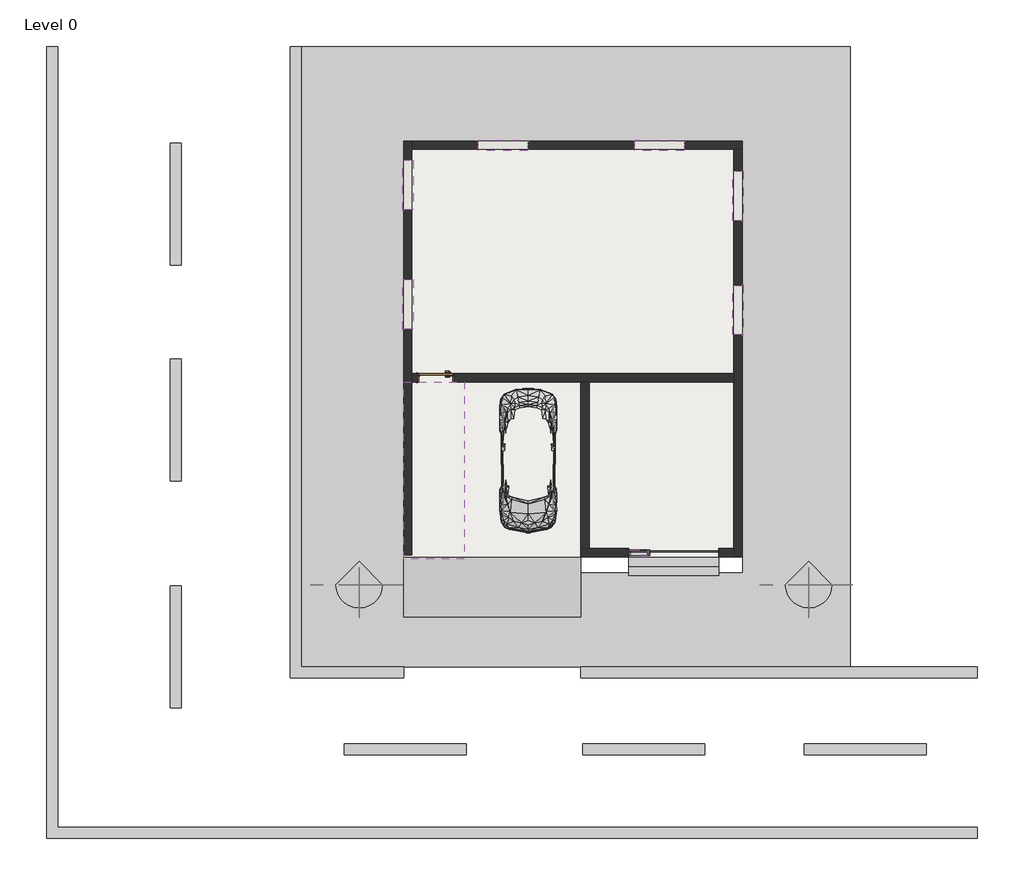
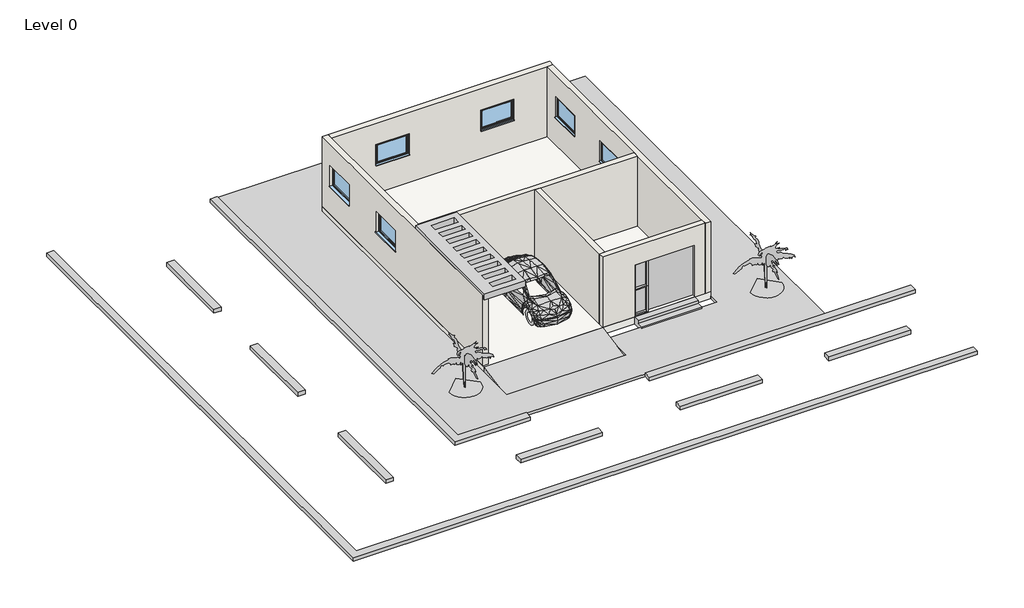
# One storey: 7 members, 6 walls, 6 windows, 4 proxies, 3 plates, 2 geographic elements, 1 door, 1 slab.
"""IFC4 building model written with IfcOpenShell, lengths in millimetres."""

from ifc_helpers import new_model, si_unit, frame, origin, origin_with_axes, place, context, project, spatial, polyline, outline, extrude, faceted_brep, transform, mapped, element, save
from components import generic_models_1_generic_models_1_b1455ff5, generic_models_4_generic_models_4_16c068d2, generic_models_5_generic_models_5_f3326099, rpc_beetle_rpc_beetle_31f8b51e, doors_intsgl_1010x2110mm_2294229c, rpc_tree_tropical_australian_tree_furn_6_77f1a640, rectangular_mullion_50x150mm_bddf6eb5, rectangular_mullion_50x150mm_e26dd5f5, rectangular_mullion_50x150mm_60451361, system_panel_glazed_79c163db, system_panel_glazed_e26c2a08, windows_sgl_plain_1360x910mm_0a0c3bd6

model = new_model("IFC4")

# Units and contexts
model_context = context("Model", 3, world=origin())
ifc_project = project(units=[si_unit("LENGTHUNIT", "METRE", prefix="MILLI")], contexts=[model_context])

# Site, building, storey
site = spatial("IfcSite", under=ifc_project)
building = spatial("IfcBuilding", under=site)
storey = spatial("IfcBuildingStorey", under=building, Name="Level 0", Elevation=0.0)

# Proxies
placement = place(None, origin())
generic_models_1_generic_models_1_shape = generic_models_1_generic_models_1_b1455ff5(model_context)
element("IfcBuildingElementProxy", 1, Name="Generic Models 1 : Generic Models 1", ObjectType="Generic Models 1 : Generic Models 1", at=placement, inside=storey, context=model_context, shape_type="MappedRepresentation", body=[
    mapped(generic_models_1_generic_models_1_shape, transform((0.0, 0.0, 0.0), x_axis=(1.0, 0.0, 0.0), y_axis=(0.0, 1.0, 0.0), z_axis=(0.0, 0.0, 1.0))),
])
generic_models_4_generic_models_4_shape = generic_models_4_generic_models_4_16c068d2(model_context)
element("IfcBuildingElementProxy", 2, Name="Generic Models 4 : Generic Models 4", ObjectType="Generic Models 4 : Generic Models 4", at=placement, inside=storey, context=model_context, shape_type="MappedRepresentation", body=[
    mapped(generic_models_4_generic_models_4_shape, transform((0.0, 0.0, 0.0), x_axis=(1.0, 0.0, 0.0), y_axis=(0.0, 1.0, 0.0), z_axis=(0.0, 0.0, 1.0))),
])
generic_models_5_generic_models_5_shape = generic_models_5_generic_models_5_f3326099(model_context)
element("IfcBuildingElementProxy", 3, Name="Generic Models 5 : Generic Models 5", ObjectType="Generic Models 5 : Generic Models 5", at=placement, inside=storey, context=model_context, shape_type="MappedRepresentation", body=[
    mapped(generic_models_5_generic_models_5_shape, transform((0.0, 0.0, 0.0), x_axis=(1.0, 0.0, 0.0), y_axis=(0.0, 1.0, 0.0), z_axis=(0.0, 0.0, 1.0))),
])
rpc_beetle_rpc_beetle_shape = rpc_beetle_rpc_beetle_31f8b51e(model_context)
element("IfcBuildingElementProxy", 4, Name="RPC Beetle : RPC Beetle", ObjectType="RPC Beetle : RPC Beetle", at=placement, inside=storey, context=model_context, shape_type="MappedRepresentation", body=[
    mapped(rpc_beetle_rpc_beetle_shape, transform((-6051.9025595, 647.0632107, 0.0), x_axis=(-1.0, 0.0, 0.0), y_axis=(0.0, -1.0, 0.0), z_axis=(0.0, 0.0, 1.0))),
])

# Door
doors_intsgl_1010x2110mm_shape = doors_intsgl_1010x2110mm_2294229c(model_context)
element("IfcDoor", 5, ObjectType="Doors_IntSgl : 1010x2110mm", at=placement, inside=storey, context=model_context, shape_type="MappedRepresentation", body=[
    mapped(doors_intsgl_1010x2110mm_shape, transform((-8594.9025595, 1694.8132107, 0.0), x_axis=(-1.0, 0.0, 0.0), y_axis=(0.0, -1.0, 0.0), z_axis=(0.0, 0.0, 1.0))),
])

# Geographic elements
rpc_tree_tropical_australian_tree_furn_6_shape = rpc_tree_tropical_australian_tree_furn_6_77f1a640(model_context)
element("IfcGeographicElement", 6, ObjectType="RPC Tree - Tropical : Australian Tree Furn - 6'", at=placement, inside=storey, context=model_context, shape_type="MappedRepresentation", body=[
    mapped(rpc_tree_tropical_australian_tree_furn_6_shape, transform((1663.3474405, -4001.1367893, 0.0), x_axis=(1.0, 0.0, 0.0), y_axis=(0.0, 1.0, 0.0), z_axis=(0.0, 0.0, 1.0))),
])
element("IfcGeographicElement", 7, ObjectType="RPC Tree - Tropical : Australian Tree Furn - 6'", at=placement, inside=storey, context=model_context, shape_type="MappedRepresentation", body=[
    mapped(rpc_tree_tropical_australian_tree_furn_6_shape, transform((-10700.1025595, -4001.1367893, 0.0), x_axis=(1.0, 0.0, 0.0), y_axis=(0.0, 1.0, 0.0), z_axis=(0.0, 0.0, 1.0))),
])

# Members
rectangular_mullion_50x150mm_shape = rectangular_mullion_50x150mm_bddf6eb5(model_context)
element("IfcMember", 8, ObjectType="Rectangular Mullion : 50x150mm", at=placement, inside=storey, context=model_context, shape_type="MappedRepresentation", body=[
    mapped(rectangular_mullion_50x150mm_shape, transform((-2757.4025595, -3124.8367893, 2250.0), x_axis=(0.0, 0.0, 1.0), y_axis=(0.0, -1.0, 0.0), z_axis=(1.0, 0.0, 0.0))),
])
element("IfcMember", 9, ObjectType="Rectangular Mullion : 50x150mm", at=placement, inside=storey, context=model_context, shape_type="MappedRepresentation", body=[
    mapped(rectangular_mullion_50x150mm_shape, transform((-3241.6025595, -3124.8367893, 0.0), x_axis=(0.0, 0.0, -1.0), y_axis=(0.0, -1.0, 0.0), z_axis=(-1.0, 0.0, 0.0))),
])
rectangular_mullion_50x150mm_2_shape = rectangular_mullion_50x150mm_e26dd5f5(model_context)
element("IfcMember", 10, ObjectType="Rectangular Mullion : 50x150mm", at=placement, inside=storey, context=model_context, shape_type="MappedRepresentation", body=[
    mapped(rectangular_mullion_50x150mm_2_shape, transform((-2757.4025595, -3124.8367893, 1125.0), x_axis=(0.0, 0.0, 1.0), y_axis=(0.0, -1.0, 0.0), z_axis=(1.0, 0.0, 0.0))),
])
rectangular_mullion_50x150mm_3_shape = rectangular_mullion_50x150mm_60451361(model_context)
element("IfcMember", 11, ObjectType="Rectangular Mullion : 50x150mm", at=placement, inside=storey, context=model_context, shape_type="MappedRepresentation", body=[
    mapped(rectangular_mullion_50x150mm_3_shape, transform((-2707.4025595, -3124.8367893, 0.0), x_axis=(1.0, 0.0, 0.0), y_axis=(0.0, -1.0, 0.0), z_axis=(0.0, 0.0, -1.0))),
])
element("IfcMember", 12, ObjectType="Rectangular Mullion : 50x150mm", at=placement, inside=storey, context=model_context, shape_type="MappedRepresentation", body=[
    mapped(rectangular_mullion_50x150mm_3_shape, transform((-3291.6025595, -3124.8367893, 2250.0), x_axis=(-1.0, 0.0, 0.0), y_axis=(0.0, -1.0, 0.0), z_axis=(0.0, 0.0, 1.0))),
])
element("IfcMember", 13, ObjectType="Rectangular Mullion : 50x150mm", at=placement, inside=storey, context=model_context, shape_type="MappedRepresentation", body=[
    mapped(rectangular_mullion_50x150mm_3_shape, transform((-2707.4025595, -3124.8367893, 1125.0), x_axis=(1.0, 0.0, 0.0), y_axis=(0.0, -1.0, 0.0), z_axis=(0.0, 0.0, -1.0))),
])
element("IfcMember", 14, ObjectType="Rectangular Mullion : 50x150mm", at=placement, inside=storey, context=model_context, shape_type="MappedRepresentation", body=[
    mapped(rectangular_mullion_50x150mm_3_shape, transform((-3291.6025595, -3124.8367893, 1125.0), x_axis=(-1.0, 0.0, 0.0), y_axis=(0.0, -1.0, 0.0), z_axis=(0.0, 0.0, 1.0))),
])

# Plates
system_panel_glazed_shape = system_panel_glazed_79c163db(model_context)
element("IfcPlate", 15, ObjectType="System Panel : Glazed", at=placement, inside=storey, context=model_context, shape_type="MappedRepresentation", body=[
    mapped(system_panel_glazed_shape, transform((-2999.5025595, -3124.8367893, 50.0), x_axis=(1.0, 0.0, 0.0), y_axis=(0.0, 1.0, 0.0), z_axis=(0.0, 0.0, 1.0))),
])
element("IfcPlate", 16, ObjectType="System Panel : Glazed", at=placement, inside=storey, context=model_context, shape_type="MappedRepresentation", body=[
    mapped(system_panel_glazed_shape, transform((-2999.5025595, -3124.8367893, 1150.0), x_axis=(1.0, 0.0, 0.0), y_axis=(0.0, 1.0, 0.0), z_axis=(0.0, 0.0, 1.0))),
])
system_panel_glazed_2_shape = system_panel_glazed_e26c2a08(model_context)
element("IfcPlate", 17, ObjectType="System Panel : Glazed", at=placement, inside=storey, context=model_context, shape_type="MappedRepresentation", body=[
    mapped(system_panel_glazed_2_shape, transform((-1762.0025595, -3124.8367893, 0.0), x_axis=(1.0, 0.0, 0.0), y_axis=(0.0, 1.0, 0.0), z_axis=(0.0, 0.0, 1.0))),
])

# Slab
element("IfcSlab", 18, ObjectType="12\" floor", at=placement, inside=storey, context=model_context, shape_type="SweptSolid", body=[
    extrude(outline(polyline([(-165.4525595, 8209.9132107), (-165.4525595, -3239.1367893), (-9480.9025595, -3239.1367893), (-9480.9025595, 8209.9132107), (-165.4525595, 8209.9132107)])), frame((0.0, 0.0, -304.8), z_axis=(0.0, 0.0, 1.0), x_axis=(1.0, 0.0, 0.0)), (0.0, 0.0, 1.0), 304.8),
])

# Walls
element("IfcWall", 19, ObjectType="9\" wall", at=placement, inside=storey, context=model_context, shape_type="Brep", body=[
    faceted_brep([(-9252.3025595, -3181.9867893, 0.0), (-9252.3025595, 1580.5132107, 0.0), (-9252.3025595, 1809.1132107, 0.0), (-9252.3025595, 7981.3132107, 0.0), (-9252.3025595, 8209.9132107, 0.0), (-9252.3025595, 8209.9132107, 3048.0), (-9252.3025595, 7981.3132107, 3048.0), (-9252.3025595, 1809.1132107, 3048.0), (-9252.3025595, 1580.5132107, 3048.0), (-9252.3025595, -3181.9867893, 3048.0), (-9252.3025595, 7676.5132107, 2110.0), (-9252.3025595, 7676.5132107, 1200.0), (-9252.3025595, 6316.5132107, 1200.0), (-9252.3025595, 6316.5132107, 2110.0), (-9252.3025595, 4388.3132107, 2110.0), (-9252.3025595, 4388.3132107, 1200.0), (-9252.3025595, 3028.3132107, 1200.0), (-9252.3025595, 3028.3132107, 2110.0), (-9480.9025595, -3181.9867893, 0.0), (-9480.9025595, -3181.9867893, 3048.0), (-9480.9025595, 8209.9132107, 3048.0), (-9480.9025595, 8209.9132107, 0.0), (-9480.9025595, 7676.5132107, 2110.0), (-9480.9025595, 6316.5132107, 2110.0), (-9480.9025595, 6316.5132107, 1200.0), (-9480.9025595, 7676.5132107, 1200.0), (-9480.9025595, 4388.3132107, 2110.0), (-9480.9025595, 3028.3132107, 2110.0), (-9480.9025595, 3028.3132107, 1200.0), (-9480.9025595, 4388.3132107, 1200.0)], [[[0, 1, 2, 3, 4, 5, 6, 7, 8, 9], [10, 11, 12, 13], [14, 15, 16, 17]], [[18, 19, 20, 21], [22, 23, 24, 25], [26, 27, 28, 29]], [[4, 3, 2, 1, 0, 18, 21]], [[9, 8, 7, 6, 5, 20, 19]], [[0, 9, 19, 18]], [[5, 4, 21, 20]], [[11, 10, 22, 25]], [[12, 11, 25, 24]], [[13, 12, 24, 23]], [[10, 13, 23, 22]], [[15, 14, 26, 29]], [[16, 15, 29, 28]], [[17, 16, 28, 27]], [[14, 17, 27, 26]]]),
])
element("IfcWall", 20, ObjectType="9\" wall", at=placement, inside=storey, context=model_context, shape_type="Brep", body=[
    faceted_brep([(-394.0525595, 1580.5132107, 3048.0), (-4375.5025595, 1580.5132107, 3048.0), (-4604.1025595, 1580.5132107, 3048.0), (-9252.3025595, 1580.5132107, 3048.0), (-9252.3025595, 1580.5132107, 0.0), (-9099.9025595, 1580.5132107, 0.0), (-9099.9025595, 1580.5132107, 2110.0), (-8089.9025595, 1580.5132107, 2110.0), (-8089.9025595, 1580.5132107, 0.0), (-4604.1025595, 1580.5132107, 0.0), (-4375.5025595, 1580.5132107, 0.0), (-394.0525595, 1580.5132107, 0.0), (-9252.3025595, 1809.1132107, 3048.0), (-394.0525595, 1809.1132107, 3048.0), (-394.0525595, 1809.1132107, 0.0), (-8089.9025595, 1809.1132107, 0.0), (-8089.9025595, 1809.1132107, 2110.0), (-9099.9025595, 1809.1132107, 2110.0), (-9099.9025595, 1809.1132107, 0.0), (-9252.3025595, 1809.1132107, 0.0)], [[[0, 1, 2, 3, 4, 5, 6, 7, 8, 9, 10, 11]], [[12, 13, 14, 15, 16, 17, 18, 19]], [[4, 19, 18, 5]], [[14, 11, 10, 9, 8, 15]], [[3, 2, 1, 0, 13, 12]], [[4, 3, 12, 19]], [[0, 11, 14, 13]], [[17, 6, 5, 18]], [[6, 17, 16, 7]], [[7, 16, 15, 8]]]),
])
element("IfcWall", 21, ObjectType="9\" wall", at=placement, inside=storey, context=model_context, shape_type="Brep", body=[
    faceted_brep([(-394.0525595, 7981.3132107, 0.0), (-394.0525595, 1809.1132107, 0.0), (-394.0525595, 1580.5132107, 0.0), (-394.0525595, -3010.5367893, 0.0), (-394.0525595, -3239.1367893, 0.0), (-394.0525595, -3239.1367893, 3048.0), (-394.0525595, -3010.5367893, 3048.0), (-394.0525595, 1580.5132107, 3048.0), (-394.0525595, 1809.1132107, 3048.0), (-394.0525595, 7981.3132107, 3048.0), (-394.0525595, 2875.9132107, 2110.0), (-394.0525595, 2875.9132107, 1200.0), (-394.0525595, 4235.9132107, 1200.0), (-394.0525595, 4235.9132107, 2110.0), (-394.0525595, 6011.7132107, 2110.0), (-394.0525595, 6011.7132107, 1200.0), (-394.0525595, 7371.7132107, 1200.0), (-394.0525595, 7371.7132107, 2110.0), (-165.4525595, 7981.3132107, 0.0), (-165.4525595, 7981.3132107, 3048.0), (-165.4525595, -3239.1367893, 3048.0), (-165.4525595, -3239.1367893, 0.0), (-165.4525595, 2875.9132107, 2110.0), (-165.4525595, 4235.9132107, 2110.0), (-165.4525595, 4235.9132107, 1200.0), (-165.4525595, 2875.9132107, 1200.0), (-165.4525595, 6011.7132107, 2110.0), (-165.4525595, 7371.7132107, 2110.0), (-165.4525595, 7371.7132107, 1200.0), (-165.4525595, 6011.7132107, 1200.0)], [[[0, 1, 2, 3, 4, 5, 6, 7, 8, 9], [10, 11, 12, 13], [14, 15, 16, 17]], [[18, 19, 20, 21], [22, 23, 24, 25], [26, 27, 28, 29]], [[4, 3, 2, 1, 0, 18, 21]], [[9, 8, 7, 6, 5, 20, 19]], [[5, 4, 21, 20]], [[0, 9, 19, 18]], [[11, 10, 22, 25]], [[12, 11, 25, 24]], [[13, 12, 24, 23]], [[10, 13, 23, 22]], [[15, 14, 26, 29]], [[16, 15, 29, 28]], [[17, 16, 28, 27]], [[14, 17, 27, 26]]]),
])
element("IfcWall", 22, ObjectType="9\" wall", at=placement, inside=storey, context=model_context, shape_type="Brep", body=[
    faceted_brep([(-394.0525595, -3010.5367893, 0.0), (-816.6025595, -3010.5367893, 0.0), (-816.6025595, -3010.5367893, 2250.0), (-3291.6025595, -3010.5367893, 2250.0), (-3291.6025595, -3010.5367893, 0.0), (-4375.5025595, -3010.5367893, 0.0), (-4604.1025595, -3010.5367893, 0.0), (-4604.1025595, -3010.5367893, 3048.0), (-4375.5025595, -3010.5367893, 3048.0), (-394.0525595, -3010.5367893, 3048.0), (-394.0525595, -3239.1367893, 0.0), (-394.0525595, -3239.1367893, 3048.0), (-4604.1025595, -3239.1367893, 3048.0), (-4604.1025595, -3239.1367893, 0.0), (-3291.6025595, -3239.1367893, 0.0), (-3291.6025595, -3239.1367893, 2250.0), (-816.6025595, -3239.1367893, 2250.0), (-816.6025595, -3239.1367893, 0.0)], [[[0, 1, 2, 3, 4, 5, 6, 7, 8, 9]], [[10, 11, 12, 13, 14, 15, 16, 17]], [[0, 9, 11, 10]], [[7, 6, 13, 12]], [[9, 8, 7, 12, 11]], [[1, 0, 10, 17]], [[2, 1, 17, 16]], [[3, 2, 16, 15]], [[4, 3, 15, 14]], [[6, 5, 4, 14, 13]]]),
])
element("IfcWall", 23, ObjectType="9\" wall", at=placement, inside=storey, context=model_context, shape_type="SweptSolid", body=[
    extrude(outline(polyline([(-4375.5025595, 1580.5132107), (-4375.5025595, -3010.5367893), (-4604.1025595, -3010.5367893), (-4604.1025595, 1580.5132107), (-4375.5025595, 1580.5132107)])), origin_with_axes(), (0.0, 0.0, 1.0), 3048.0),
])
element("IfcWall", 24, ObjectType="9\" wall", at=placement, inside=storey, context=model_context, shape_type="Brep", body=[
    faceted_brep([(-9252.3025595, 7981.3132107, 0.0), (-394.0525595, 7981.3132107, 0.0), (-165.4525595, 7981.3132107, 0.0), (-165.4525595, 7981.3132107, 3048.0), (-394.0525595, 7981.3132107, 3048.0), (-9252.3025595, 7981.3132107, 3048.0), (-1765.6525595, 7981.3132107, 2110.0), (-1765.6525595, 7981.3132107, 1200.0), (-3125.6525595, 7981.3132107, 1200.0), (-3125.6525595, 7981.3132107, 2110.0), (-6063.5025595, 7981.3132107, 2110.0), (-6063.5025595, 7981.3132107, 1200.0), (-7423.5025595, 7981.3132107, 1200.0), (-7423.5025595, 7981.3132107, 2110.0), (-9252.3025595, 8209.9132107, 0.0), (-9252.3025595, 8209.9132107, 3048.0), (-165.4525595, 8209.9132107, 3048.0), (-165.4525595, 8209.9132107, 0.0), (-1765.6525595, 8209.9132107, 2110.0), (-3125.6525595, 8209.9132107, 2110.0), (-3125.6525595, 8209.9132107, 1200.0), (-1765.6525595, 8209.9132107, 1200.0), (-6063.5025595, 8209.9132107, 2110.0), (-7423.5025595, 8209.9132107, 2110.0), (-7423.5025595, 8209.9132107, 1200.0), (-6063.5025595, 8209.9132107, 1200.0)], [[[0, 1, 2, 3, 4, 5], [6, 7, 8, 9], [10, 11, 12, 13]], [[14, 15, 16, 17], [18, 19, 20, 21], [22, 23, 24, 25]], [[2, 1, 0, 14, 17]], [[5, 4, 3, 16, 15]], [[0, 5, 15, 14]], [[3, 2, 17, 16]], [[7, 6, 18, 21]], [[8, 7, 21, 20]], [[9, 8, 20, 19]], [[6, 9, 19, 18]], [[11, 10, 22, 25]], [[12, 11, 25, 24]], [[13, 12, 24, 23]], [[10, 13, 23, 22]]]),
])

# Windows
windows_sgl_plain_1360x910mm_shape = windows_sgl_plain_1360x910mm_0a0c3bd6(model_context)
element("IfcWindow", 25, ObjectType="Windows_Sgl_Plain : 1360x910mm", at=placement, inside=storey, context=model_context, shape_type="MappedRepresentation", body=[
    mapped(windows_sgl_plain_1360x910mm_shape, transform((-271.2959916, 3555.9132107, 0.0), x_axis=(0.0, 1.0, 0.0), y_axis=(-1.0, 0.0, 0.0), z_axis=(0.0, 0.0, 1.0))),
])
element("IfcWindow", 26, ObjectType="Windows_Sgl_Plain : 1360x910mm", at=placement, inside=storey, context=model_context, shape_type="MappedRepresentation", body=[
    mapped(windows_sgl_plain_1360x910mm_shape, transform((-271.2959916, 6691.7132107, 0.0), x_axis=(0.0, 1.0, 0.0), y_axis=(-1.0, 0.0, 0.0), z_axis=(0.0, 0.0, 1.0))),
])
element("IfcWindow", 27, ObjectType="Windows_Sgl_Plain : 1360x910mm", at=placement, inside=storey, context=model_context, shape_type="MappedRepresentation", body=[
    mapped(windows_sgl_plain_1360x910mm_shape, transform((-2445.6525595, 8104.0697785, 0.0), x_axis=(-1.0, 0.0, 0.0), y_axis=(0.0, -1.0, 0.0), z_axis=(0.0, 0.0, 1.0))),
])
element("IfcWindow", 28, ObjectType="Windows_Sgl_Plain : 1360x910mm", at=placement, inside=storey, context=model_context, shape_type="MappedRepresentation", body=[
    mapped(windows_sgl_plain_1360x910mm_shape, transform((-6743.5025595, 8104.0697785, 0.0), x_axis=(-1.0, 0.0, 0.0), y_axis=(0.0, -1.0, 0.0), z_axis=(0.0, 0.0, 1.0))),
])
element("IfcWindow", 29, ObjectType="Windows_Sgl_Plain : 1360x910mm", at=placement, inside=storey, context=model_context, shape_type="MappedRepresentation", body=[
    mapped(windows_sgl_plain_1360x910mm_shape, transform((-9375.0591273, 6996.5132107, 0.0), x_axis=(0.0, -1.0, 0.0), y_axis=(1.0, 0.0, 0.0), z_axis=(0.0, 0.0, 1.0))),
])
element("IfcWindow", 30, ObjectType="Windows_Sgl_Plain : 1360x910mm", at=placement, inside=storey, context=model_context, shape_type="MappedRepresentation", body=[
    mapped(windows_sgl_plain_1360x910mm_shape, transform((-9375.0591273, 3708.3132107, 0.0), x_axis=(0.0, -1.0, 0.0), y_axis=(1.0, 0.0, 0.0), z_axis=(0.0, 0.0, 1.0))),
])

save(model, "model.ifc")

# Revit data of these elements
# Type "RPC Beetle : RPC Beetle"
#   built-in parameter 1005198 = "{2, 15},{39, RPC-16-0U6E-L4EG-ENH1-J3KF-SVEL-0TX4-C0},{1, 0},{1, 0},{2, 36},{1, 8},{5, Color},{1, 0},{1, 0},{3, 0.8},{3, 0.8},{3, 0.8},{1, 8},{7, BBoxMin},{1, 0},{1, 0},{1, 0},{1, 0},{1, 0},{1, 8},{7, BBoxMax},{1, 0},{1, 0},{1, 0},{1, 0},{1, 0},{2, 11},{9, RPCTypeId},{1, 0},{1, 0},{39, RPC-16-0U6E-L4EG-ENH1-J3KF-SVEL-0TX4-C0},{1, 6},{14, RPCPlantHeight},{1, 0},{1, 0},{7, 4.91667},{2, 11},{20, AdvancedUIDefinition},{1, 0},{1, 0},{0, },{2, 11},{10, AssetLibID},{1, 0},{1, 0},{36, 4D3F6E72-3F99-4203-98E9-AF80B3C7A7A4},{2, 11},{10, BaseSchema},{1, 0},{1, 0},{9, RPCSchema},{2, 11},{12, ExchangeGUID},{1, 0},{1, 0},{0, },{1, 2},{6, Hidden},{1, 0},{1, 0},{1, 0},{2, 11},{12, LocalizedUID},{1, 0},{1, 0},{0, },{1, 4},{11, RPCCategory},{1, 0},{1, 0},{1, 0},{2, 11},{8, RPCImage},{1, 0},{1, 0},{0, },{1, 4},{13, SchemaVersion},{1, 0},{1, 0},{1, 4},{2, 11},{12, UIDefinition},{1, 0},{1, 0},{0, },{2, 11},{6, UIName},{1, 0},{1, 0},{39, RPC-16-0U6E-L4EG-ENH1-J3KF-SVEL-0TX4-C0},{2, 11},{11, VersionGUID},{1, 0},{1, 0},{9, RPCSchema},{2, 11},{9, assettype},{1, 0},{1, 0},{11, RPCGeometry},{2, 11},{11, description},{1, 0},{1, 0},{0, },{2, 11},{9, localname},{1, 0},{1, 0},{3, RPC},{2, 11},{9, localtype},{1, 0},{1, 0},{3, RPC},{1, 4},{8, revision},{1, 0},{1, 0},{1, 1},{2, 11},{9, thumbnail},{1, 0},{1, 0},{0, },{1, 4},{7, version},{1, 0},{1, 0},{1, 1},{2, 14},{6, Height},{1, 0},{1, 0},{7, 4.91667},{1, 2},{20, RPC_Cast Reflections},{1, 0},{1, 0},{1, 1},{1, 4},{16, RPC_Transparency},{1, 0},{1, 0},{2, 18},{1, 4},{11, RPC_Tinting},{1, 0},{1, 0},{2, 50},{1, 2},{15, RPC_Use Tinting},{1, 0},{1, 0},{1, 0},{1, 2},{17, RPC_License Plate},{1, 0},{1, 0},{1, 0},{2, 11},{25, RPC_License Plate Texture},{1, 0},{1, 0},{64, __RPC:/object data/textures/car/plate/textures/default/rgb/0/0/0},{2, 11},{27, RPC_i_License Plate Texture},{1, 0},{1, 0},{0, },{1, 2},{16, RPC_Custom Plate},{1, 0},{1, 0},{1, 0},{2, 11},{27, RPC_License Plate File Name},{1, 0},{1, 0},{0, },{2, 11},{7, keyword},{1, 0},{1, 0},{27, :Geometry:RPC:VW Beetle [4]},{2, 11},{8, category},{1, 0},{1, 0},{21, :Auto_Economy/Midsize},{21, assetlibrary_base.fbx},{1, 5},"
#   built-in parameter 1005195 = "RPC-16-0U6E-L4EG-ENH1-J3KF-SVEL-0TX4-C0"
#   Height = 0
# Type "Doors_IntSgl : 1010x2110mm"
#   Construction Type Id = "MDOOR"
#   Type Mark = "43"
#   Type Comments = "Internal Single"
#   Operation = "SingleSwingRight"
#   Manufacturer = "Revit"
#   Keynote = "L20"
#   Description = "Internal Single Door"
#   Analytic Construction = "Metal"
#   UnderCut = 8 mm
#   Tolerance = 2 mm
#   Thickness = 38 mm
#   Thermal Resistance (R) = 0.270117 (m²·K)/W
#   Structural Tolerance = 8 mm
#   StopDepth = 32 mm
#   Stop Thickness = 19 mm
#   Rough Width = 1010 mm
#   Rough Height = 2110 mm
#   Height to Top Lock Rail = 1000 mm
#   Heat Transfer Coefficient (U) = 3.7021 W/(m²·K)
#   Handle Z Distance = 900 mm
#   Handle X Distance = 75 mm
#   Frame Thickness = 32 mm
#   Door Panel Width = 926 mm
#   Door Panel Thickness = 38 mm
#   Door Panel Offset = 0 mm
#   Height = 2110 mm
#   Width = 1010 mm
#   Door Panel Height = 2060 mm
#   Architrave Setback = 5 mm
#   Define Thermal Properties by = 1
#   Vis - Ironmongery = yes
#   Material Ironmongery = Door - Handle
#   Material Frame = Door - Frame/Mullion (1)
#   Material Door = Door - Panel
#   Material Architrave = Door - Architrave
#   Visual Light Transmittance = 0
#   Solar Heat Gain Coefficient = 0
#   Function = (empty or 0)
#   Wall Closure = (empty or 0)
# Type "RPC Tree - Tropical : Australian Tree Furn - 6'"
#   built-in parameter 1005198 = "{2, 15},{39, RPC-16-FVCN-UWG0-AP53-A000-ST1L-LVER-AU},{1, 0},{1, 0},{2, 35},{1, 8},{5, Color},{1, 0},{1, 0},{3, 0.8},{3, 0.8},{3, 0.8},{1, 8},{7, BBoxMin},{1, 0},{1, 0},{1, 0},{1, 0},{1, 0},{1, 8},{7, BBoxMax},{1, 0},{1, 0},{1, 0},{1, 0},{1, 0},{2, 11},{9, RPCTypeId},{1, 0},{1, 0},{39, RPC-16-FVCN-UWG0-AP53-A000-ST1L-LVER-AU},{1, 6},{14, RPCPlantHeight},{1, 0},{1, 0},{1, 6},{2, 11},{7, keyword},{1, 0},{1, 0},{99, :Geometry:RPC:Australian Tree Fern:Alsophila cooperi (Cyathea australis):Sydney:Tree fern:Tropical.},{2, 11},{8, category},{1, 0},{1, 0},{17, :Trees [Tropical]},{2, 11},{12, LocalizedUID},{1, 0},{1, 0},{20, Australian Tree Fern},{2, 14},{6, Height},{1, 0},{1, 0},{1, 6},{1, 2},{16, Cast Reflections},{1, 0},{1, 0},{1, 0},{1, 2},{12, Cast Shadows},{1, 0},{1, 0},{1, 1},{1, 2},{9, Lock View},{1, 0},{1, 0},{1, 0},{1, 4},{5, ViewC},{1, 0},{1, 0},{1, 0},{2, 11},{20, AdvancedUIDefinition},{1, 0},{1, 0},{0, },{2, 11},{10, AssetLibID},{1, 0},{1, 0},{36, 4D3F6E72-3F99-4203-98E9-AF80B3C7A7A4},{2, 11},{10, BaseSchema},{1, 0},{1, 0},{9, RPCSchema},{2, 11},{12, ExchangeGUID},{1, 0},{1, 0},{0, },{1, 2},{6, Hidden},{1, 0},{1, 0},{1, 0},{1, 4},{11, RPCCategory},{1, 0},{1, 0},{1, 0},{2, 11},{8, RPCImage},{1, 0},{1, 0},{0, },{1, 4},{13, SchemaVersion},{1, 0},{1, 0},{1, 4},{2, 11},{12, UIDefinition},{1, 0},{1, 0},{0, },{2, 11},{6, UIName},{1, 0},{1, 0},{39, RPC-16-FVCN-UWG0-AP53-A000-ST1L-LVER-AU},{2, 11},{11, VersionGUID},{1, 0},{1, 0},{9, RPCSchema},{2, 11},{9, assettype},{1, 0},{1, 0},{11, RPCGeometry},{2, 11},{11, description},{1, 0},{1, 0},{0, },{2, 11},{9, localname},{1, 0},{1, 0},{3, RPC},{2, 11},{9, localtype},{1, 0},{1, 0},{3, RPC},{1, 4},{8, revision},{1, 0},{1, 0},{1, 1},{2, 11},{9, thumbnail},{1, 0},{1, 0},{0, },{1, 4},{7, version},{1, 0},{1, 0},{1, 1},{1, 2},{20, RPC_Cast Reflections},{1, 0},{1, 0},{1, 1},{1, 2},{16, RPC_Cast Shadows},{1, 0},{1, 0},{1, 1},{1, 2},{13, RPC_Lock View},{1, 0},{1, 0},{1, 0},{1, 4},{9, RPC_ViewC},{1, 0},{1, 0},{1, 0},{21, assetlibrary_base.fbx},{1, 5},"
#   built-in parameter 1005195 = "RPC-16-FVCN-UWG0-AP53-A000-ST1L-LVER-AU"
#   Type Comments = "Australian Tree Furn"
#   Assembly Code = "G2050500"
#   Height = 1828.8 mm
#   Plan Symbol = element 336060
#   Default Elevation = 0
# Type "Rectangular Mullion : 50x150mm"
#   Keynote = "H11"
#   built-in parameter 1007304 = 0.492126 (stored number, unit not read)
#   built-in parameter 1007301 = 0.082021 (stored number, unit not read)
#   built-in parameter 1007300 = 0.082021 (stored number, unit not read)
# Type "System Panel : Glazed"
#   Keynote = "H11"
#   Construction Type Id = "GSP4R"
#   Analytic Construction = "1/8 in Pilkington single glazing"
#   Visual Light Transmittance = 0.9
#   Solar Heat Gain Coefficient = 0.86
#   Heat Transfer Coefficient (U) = 6.7069 W/(m²·K)
#   Define Thermal Properties by = 1
# Type "12\" floor"
#   Keynote = "E60/130"
#   Function = 0
#   Layers, outside or top first: 304.8 mm "Concrete, Precast" (function 1)
# Type "9\" wall"
#   Keynote = "F10"
#   Layers, outside or top first: 228.6 mm "Concrete Masonry Units _Low Density" (function 1)
# Type "Windows_Sgl_Plain : 1360x910mm"
#   Type Mark = "46"
#   Operation = "SinglePanel"
#   Construction Type Id = "SGL"
#   Manufacturer = "Revit"
#   Keynote = "L10"
#   Analytic Construction = "Large single-glazed windows"
#   Wrap Layers (Ext) from Ext = 102.5 mm
#   Wrap Layers (Int) from Ext = 177.5 mm
#   Window Board Projection = 25 mm
#   Window Board Extension = 25 mm
#   Visual Light Transmittance = 0.9
#   Solar Heat Gain Coefficient = 0.86
#   Rough Width = 1360 mm
#   Rough Height = 910 mm
#   Height = 910 mm
#   Width = 1360 mm
#   Heat Transfer Coefficient (U) = 5.5617 W/(m²·K)
#   Glazing Thickness = 24 mm
#   FrameOffset - External = 50 mm
#   Frame Depth = 65 mm
#   Default Head Height = 2110 mm
#   Cill Depth = 87.5 mm
#   Cavity Closer Width = 50 mm
#   Cavity Closer Offset from Ext = 102.5 mm
#   Cavity Closer Depth = 85 mm
#   Define Thermal Properties by = 1
#   Vis - Cavity Closers = yes
#   Define Thermal Properties by = 1
#   Material Trim = Window Frame
#   Material Glass = Glass
#   Material Frame = Window Frame
#   Wall Closure = (empty or 0)
# Element 1 (IfcBuildingElementProxy, "Generic Models 1 : Generic Models 1")
#   Phase Created = New Construction
# Element 2 (IfcBuildingElementProxy, "Generic Models 4 : Generic Models 4")
#   Phase Created = New Construction
# Element 3 (IfcBuildingElementProxy, "Generic Models 5 : Generic Models 5")
#   Phase Created = New Construction
#   Materials on its faces: "Gypsum Wall Board"
# Element 4 (IfcBuildingElementProxy, "RPC Beetle : RPC Beetle")
#   Phase Created = New Construction
# Element 5 (IfcDoor, "Doors_IntSgl : 1010x2110mm")
#   Phase Created = New Construction
#   Materials on its faces: "Door - Architrave", "Door - Handle", "Door - Frame/Mullion (1)", "Door - Panel"
# Elements 6, 7 (IfcGeographicElement, "RPC Tree - Tropical : Australian Tree Furn - 6'")
#   Phase Created = New Construction
# Elements 8, 9, 10, 11, 12, 13, 14 (IfcMember, "Rectangular Mullion : 50x150mm")
#   Phase Created = New Construction
#   Materials on its faces: "Aluminium"
# Elements 15, 16, 17 (IfcPlate, "System Panel : Glazed")
#   Phase Created = New Construction
#   Materials on its faces: "Glass"
# Element 18 (IfcSlab, "12\" floor")
#   Height Offset From Level = 0 mm
#   Phase Created = New Construction
#   Materials on its faces: "Concrete, Precast", "floor"
# Elements 19, 23, 24 (IfcWall, "9\" wall")
#   Top Offset = 0 mm
#   Base Offset = 0 mm
#   wall height = 3048 mm
#   Phase Created = New Construction
#   Base Constraint = Level 0
#   Top Constraint = Level 1
#   Materials on its faces: "Concrete Masonry Units _Low Density"
# Elements 20, 21, 22 (IfcWall, "9\" wall")
#   Top Offset = 0 mm
#   Base Offset = 0 mm
#   wall height = 3048 mm
#   Phase Created = New Construction
#   Base Constraint = Level 0
#   Top Constraint = Level 1
#   Materials on its faces: "Concrete Masonry Units _Low Density", "face"
# Element 25 (IfcWindow, "Windows_Sgl_Plain : 1360x910mm")
#   Mark = "4"
#   Phase Created = New Construction
#   Materials on its faces: "Window Frame", "Glass"
# Element 26 (IfcWindow, "Windows_Sgl_Plain : 1360x910mm")
#   Mark = "5"
#   Phase Created = New Construction
#   Materials on its faces: "Window Frame", "Glass"
# Element 27 (IfcWindow, "Windows_Sgl_Plain : 1360x910mm")
#   Mark = "6"
#   Phase Created = New Construction
#   Materials on its faces: "Window Frame", "Glass"
# Element 28 (IfcWindow, "Windows_Sgl_Plain : 1360x910mm")
#   Mark = "7"
#   Phase Created = New Construction
#   Materials on its faces: "Window Frame", "Glass"
# Element 29 (IfcWindow, "Windows_Sgl_Plain : 1360x910mm")
#   Mark = "8"
#   Phase Created = New Construction
#   Materials on its faces: "Window Frame", "Glass"
# Element 30 (IfcWindow, "Windows_Sgl_Plain : 1360x910mm")
#   Mark = "9"
#   Phase Created = New Construction
#   Materials on its faces: "Window Frame", "Glass"
# Materials
#   "Door - Handle": colour RGB 0 0 0, transparency 0, Keynote = "P21", Cost = 0
#   "Door - Frame/Mullion (1)": class "Wood", colour RGB 212 179 113, transparency 0, Keynote = "L20", Cost = 0
#   "Door - Panel": class "Wood", colour RGB 210 159 95, transparency 0, Keynote = "L20", Cost = 0
#   "Door - Architrave": class "Wood", colour RGB 154 90 5, transparency 0, Keynote = "P20", Cost = 0
#   "Concrete, Precast": class "Concrete", colour RGB 192 192 192, transparency 0, Description = "Precast concrete", Cost = 0
#   "Concrete Masonry Units _Low Density": class "Masonry", colour RGB 181 181 181, transparency 0, Description = "Concrete masonry units", Cost = 0
#   "Window Frame": colour RGB 249 249 249, transparency 0, Keynote = "L10", Cost = 0
#   "Glass": class "Glass", colour RGB 0 128 192, transparency 0.9, Description = "Soda Lime Glass", Cost = 0
#   "Gypsum Wall Board": class "Generic", colour RGB 228 228 228, transparency 0, Description = "Gypsum Wall Board", Cost = 0
#   "Aluminium": class "Metal", colour RGB 247 247 247, transparency 0, Description = "Aluminium 6061", Cost = 0
#   "floor": class "Generic", colour RGB 191 184 146, transparency 0, Cost = 0
#   "face": class "Generic", colour RGB 67 30 18, transparency 0, Cost = 0
